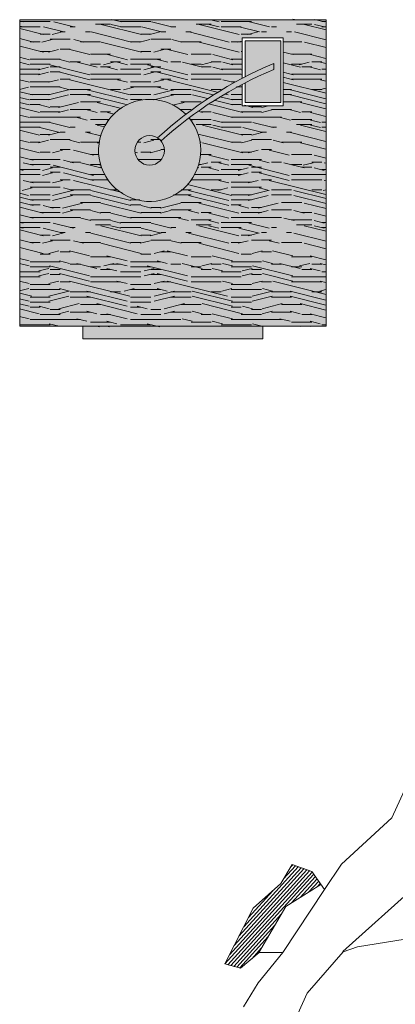
# Model space of a CAD drawing. Units: inches. Extents: x 1994 to 3075, y 3517 to 3950.
# Tile 34 of 58: x 1994.60824 to 1994.62882, y 3553.72103 to 3553.77497. Entities that reach past the tile are written whole.
import ezdxf

# ---------------------------------------------------------------- set-up
doc = ezdxf.new("R2010")
doc.units = ezdxf.units.IN
doc.layers.add('A-FURN-REFR', color=8, linetype='Continuous', lineweight=13)
doc.layers.add('A-FURN-REFR-PATT', color=8, linetype='Continuous', lineweight=13)

msp = doc.modelspace()

# ---------------------------------------------------------------- hatches: boundary and pattern name
at = {"layer": 'A-FURN-REFR-PATT'}
h = msp.add_hatch(color=256, dxfattribs=at)
h.paths.add_polyline_path([(1994.625025567844, 3553.774969762488), (1994.6082427092, 3553.774969762488), (1994.6082427092, 3553.758186903844), (1994.625025567844, 3553.758186903844)])
h.paths.add_polyline_path([(1994.617341065591, 3553.769785957469, -0.0420861834985648), (1994.620421545473, 3553.771753961409), (1994.620421545473, 3553.771757928811), (1994.620421545473, 3553.7739809259), (1994.622678150124, 3553.7739809259), (1994.622678150124, 3553.770259509415), (1994.620421545473, 3553.770259509415), (1994.620421545473, 3553.771423035513, 0.0395152736214861), (1994.617519187378, 3553.769589737948, -42.19598506456882)], flags=16)
h.paths.add_polyline_path([(1994.616171336827, 3553.767809896967, -1), (1994.614551403261, 3553.767809896967, -1)], flags=0)
h = msp.add_hatch(dxfattribs=at)
h.set_pattern_fill('LEGNO1', color=256, scale=0.005511811023622, style=0, pattern_type=2)
h.set_pattern_definition([(0, (2000.713136654079, 3549.954056641144), (0, 0.005511811023622), [0.0011023622047244, -0.0016535433070866, 0.0005511811023622, -0.0022047244094488]), (0, (2000.716994921796, 3549.95419443642), (0, 0.005511811023622), [0.0011023622047244, -0.0044094488188976]), (0, (2000.716443740693, 3549.954470026972), (0, 0.005511811023622), [0.0005511811023622, -0.0049606299212598]), (0, (2000.71341224463, 3549.954607822247), (0, 0.005511811023622), [0.0002755905511811, -0.0038582677165354, 0.0002755905511811, -0.0011023622047244]), (0, (2000.715341378489, 3549.954883412798), (0, 0.005511811023622), [0.0011023622047244, -0.0016535433070866, 0.0002755905511811, -0.0024803149606299]), (0, (2000.713963425733, 3549.955021208074), (0, 0.005511811023622), [0.0008267716535433, -0.0046850393700787]), (0, (2000.715341378489, 3549.955159003349), (0, 0.005511811023622), [0.0016535433070866, -0.0038582677165354]), (0, (2000.713687835181, 3549.955296798625), (0, 0.005511811023622), [0.0011023622047244, -0.0044094488188976]), (0, (2000.715892559591, 3549.955434593901), (0, 0.005511811023622), [0.002755905511811, -0.002755905511811]), (0, (2000.714239016284, 3549.955710184451), (0, 0.005511811023622), [0.0005511811023622, -0.0016535433070866, 0.0011023622047244, -0.0022047244094488]), (0, (2000.718097284, 3549.955847979727), (0, 0.005511811023622), [0.0011023622047244, -0.0044094488188976]), (0, (2000.716994921796, 3549.955985775002), (0, 0.005511811023622), [0.0005511811023622, -0.0049606299212598]), (0, (2000.715892559591, 3549.956123570279), (0, 0.005511811023622), [0.0005511811023622, -0.0049606299212598]), (0, (2000.713136654079, 3549.956261365553), (0, 0.005511811023622), [0.0011023622047244, -0.0044094488188976]), (0, (2000.715892559591, 3549.956399160829), (0, 0.005511811023622), [0.0011023622047244, -0.0044094488188976]), (0, (2000.715892559591, 3549.95667475138), (0, 0.005511811023622), [0.0011023622047244, -0.0011023622047244, 0.0011023622047244, -0.0022047244094488]), (0, (2000.714790197386, 3549.956950341932), (0, 0.005511811023622), [0.0005511811023622, -0.002755905511811, 0.0011023622047244, -0.0011023622047244]), (0, (2000.715892559591, 3549.957088137207), (0, 0.005511811023622), [0.0016535433070866, -0.0038582677165354]), (0, (2000.715892559591, 3549.957363727759), (0, 0.005511811023622), [0.0011023622047244, -0.0044094488188976]), (0, (2000.713687835181, 3549.957501523034), (0, 0.005511811023622), [0.0016535433070866, -0.0022047244094488, 0.0005511811023622, -0.0011023622047244]), (0, (2000.713687835181, 3549.957777113585), (0, 0.005511811023622), [0.002755905511811, -0.002755905511811]), (0, (2000.716994921796, 3549.957914908861), (0, 0.005511811023622), [0.0005511811023622, -0.0049606299212598]), (0, (2000.715341378489, 3549.958052704136), (0, 0.005511811023622), [0.0011023622047244, -0.0044094488188976]), (0, (2000.714239016284, 3549.958190499412), (0, 0.005511811023622), [0.0005511811023622, -0.0022047244094488, 0.0005511811023622, -0.0022047244094488]), (0, (2000.713687835181, 3549.958328294688), (0, 0.005511811023622), [0.0005511811023622, -0.0016535433070866, 0.0011023622047244, -0.0022047244094488]), (0, (2000.714790197386, 3549.958466089964), (0, 0.005511811023622), [0.0005511811023622, -0.002755905511811, 0.0005511811023622, -0.0016535433070866]), (0, (2000.715892559591, 3549.958603885239), (0, 0.005511811023622), [0.0016535433070866, -0.0038582677165354]), (0, (2000.713687835181, 3549.95887947579), (0, 0.005511811023622), [0.0011023622047244, -0.0044094488188976]), (0, (2000.716443740693, 3549.959017271066), (0, 0.005511811023622), [0.0005511811023622, -0.0049606299212598]), (0, (2000.717546102898, 3549.959155066341), (0, 0.005511811023622), [0.0005511811023622, -0.0049606299212598]), (14.03624347, (2000.716994921796, 3549.954470026972), (0.0055118110234648, -2.016e-13), [0.0005677165354331, -0.0221580619543307]), (14.03624347, (2000.717546102898, 3549.955710184451), (0.0055118110234648, -2.016e-13), [0.0005677165354331, -0.0221580619543307]), (14.03624347, (2000.716994921796, 3549.959017271066), (0.0055118110234648, -2.016e-13), [0.0005677165354331, -0.0221580619543307]), (14.03624347, (2000.715341378489, 3549.956950341932), (0.0055118110234648, -2.016e-13), [0.0005677165354331, -0.0221580619543307]), (14.03624347, (2000.716443740693, 3549.957777113585), (0.0055118110234648, -2.016e-13), [0.0005677165354331, -0.0221580619543307]), (14.03624347, (2000.716994921796, 3549.957363727759), (0.0055118110234648, -2.016e-13), [0.0005677165354331, -0.0221580619543307]), (14.03624347, (2000.714239016284, 3549.958328294688), (0.0055118110234648, -2.016e-13), [0.0005677165354331, -0.0221580619543307]), (14.03624347, (2000.716443740693, 3549.958052704136), (0.0055118110234648, -2.016e-13), [0.0005677165354331, -0.0221580619543307]), (14.03624347, (2000.717546102898, 3549.955985775002), (0.0055118110234648, -2.016e-13), [0.0011354330708661, -0.0215903454188977]), (14.03624347, (2000.716994921796, 3549.956399160829), (0.0055118110234648, -2.016e-13), [0.0011354330708661, -0.0215903454188977]), (14.03624347, (2000.716994921796, 3549.95667475138), (0.0055118110234648, -2.016e-13), [0.0011354330708661, -0.0215903454188977]), (165.96375653, (2000.715341378489, 3549.954883412798), (-0.0055118110234648, -2.016e-13), [0.0005677165354331, -0.0011354330708661, 0.0005677165354331, -0.0204549123480315]), (165.96375653, (2000.714239016284, 3549.955710184451), (-0.0055118110234648, -2.016e-13), [0.0005677165354331, -0.0221580619543307]), (165.96375653, (2000.714239016284, 3549.958190499412), (-0.0055118110234648, -2.016e-13), [0.0011354330708661, -0.0215903454188977]), (194.03624347, (2000.716994921796, 3549.95419443642), (-0.0055118110234648, 2.016e-13), [0.0005677165354331, -0.0221580619543307]), (345.96375653, (2000.718097284, 3549.95419443642), (0.0055118110234648, 2.016e-13), [0.0005677165354331, -0.0221580619543307]), (345.96375653, (2000.716443740693, 3549.956123570279), (0.0055118110234648, 2.016e-13), [0.0005677165354331, -0.0221580619543307]), (345.96375653, (2000.717546102898, 3549.957088137207), (0.0055118110234648, 2.016e-13), [0.0005677165354331, -0.0221580619543307]), (345.96375653, (2000.715341378489, 3549.957501523034), (0.0055118110234648, 2.016e-13), [0.0005677165354331, -0.0221580619543307]), (345.96375653, (2000.714790197386, 3549.958190499412), (0.0055118110234648, 2.016e-13), [0.0005677165354331, -0.0221580619543307]), (345.96375653, (2000.715341378489, 3549.958466089964), (0.0055118110234648, 2.016e-13), [0.0005677165354331, -0.0221580619543307]), (345.96375653, (2000.715341378489, 3549.957501523034), (0.0055118110234648, 2.016e-13), [0.0005677165354331, -0.0221580619543307]), (345.96375653, (2000.716994921796, 3549.958328294688), (0.0055118110234648, 2.016e-13), [0.0022708661417323, -0.0204549123480315]), (345.96375653, (2000.713687835181, 3549.954607822247), (0.0055118110234648, 2.016e-13), [0.0022708661417323, -0.0204549123480315]), (345.96375653, (2000.714239016284, 3549.955021208074), (0.0055118110234648, 2.016e-13), [0.0022708661417323, -0.0204549123480315]), (345.96375653, (2000.714790197386, 3549.955296798625), (0.0055118110234648, 2.016e-13), [0.0005677165354331, -0.0011354330708661, 0.0011354330708661, -0.0198871958125984]), (345.96375653, (2000.714790197386, 3549.955710184451), (0.0055118110234648, 2.016e-13), [0.0011354330708661, -0.0011354330708661, 0.0011354330708661, -0.0193194792771654]), (345.96375653, (2000.714239016284, 3549.956261365553), (0.0055118110234648, 2.016e-13), [0.0022708661417323, -0.0204549123480315]), (345.96375653, (2000.713687835181, 3549.95667475138), (0.0055118110234648, 2.016e-13), [0.0022708661417323, -0.0204549123480315]), (345.96375653, (2000.713687835181, 3549.956950341932), (0.0055118110234648, 2.016e-13), [0.0022708661417323, -0.0204549123480315]), (345.96375653, (2000.717546102898, 3549.958603885239), (0.0055118110234648, 2.016e-13), [0.0005677165354331, -0.0221580619543307]), (345.9637675300001, (2000.718097284, 3549.959155066341), (0.0055118110234647, 1.0583933e-09), [0.0011354330708661, -0.0215903454188977]), (345.9637675300001, (2000.714790197386, 3549.95887947579), (0.0055118110234647, 1.0583933e-09), [0.0011354330708661, -0.0215903454188977]), (345.96375753, (2000.714239016284, 3549.954056641144), (0.0055118110234648, 9.64008e-11), [0.0022708661417323, -0.0204549123480315]), (345.96375753, (2000.717546102898, 3549.957914908861), (0.0055118110234648, 9.64008e-11), [0.0017031496062992, -0.0210226288834646]), (345.96375753, (2000.718097284, 3549.957501523034), (0.0055118110234648, 9.64008e-11), [0.0034062992125984, -0.0193194792771654])])
h.paths.add_polyline_path([(1994.625025567844, 3553.774969762488), (1994.6082427092, 3553.774969762488), (1994.6082427092, 3553.758186903844), (1994.625025567844, 3553.758186903844)])
h.paths.add_polyline_path([(1994.617341065591, 3553.769785957469, -0.0420861834985648), (1994.620421545473, 3553.771753961409), (1994.620421545473, 3553.771757928811), (1994.620421545473, 3553.7739809259), (1994.622678150124, 3553.7739809259), (1994.622678150124, 3553.770259509415), (1994.620421545473, 3553.770259509415), (1994.620421545473, 3553.771423035513, 0.0395152736214861), (1994.617519187378, 3553.769589737948, -42.19598506456882)], flags=16)
h.paths.add_polyline_path([(1994.616171336827, 3553.767809896967, -1), (1994.614551403261, 3553.767809896967, -1)], flags=0)
msp.add_hatch(color=256, dxfattribs=at).paths.add_polyline_path([(1994.622545408993, 3553.773803717286), (1994.620598534099, 3553.773803717286), (1994.620598534099, 3553.771846057998, -0.0198106445216934), (1994.622160689546, 3553.772573101428), (1994.622160689546, 3553.772242175532, 0.0198106445217016), (1994.620598534099, 3553.771515132102), (1994.620598534099, 3553.770436718028), (1994.622545408993, 3553.770436718028)])
h = msp.add_hatch(color=256, dxfattribs=at)
h.dxf.hatch_style = 1
h.set_gradient(color1=(167, 169, 175), one_color=1, tint=1)
h.paths.add_polyline_path([(1994.622160689546, 3553.772242175532), (1994.622160689546, 3553.772573101428, 0.0875286051314429), (1994.61580001797, 3553.768490803852, -0.0763380806476787), (1994.615984121085, 3553.768327803648, -0.0846435149619904)])
h = msp.add_hatch(color=256, dxfattribs=at)
h.dxf.hatch_style = 1
h.set_gradient(color1=(37, 53, 157), color2=(142, 207, 230), tint=1, name='SPHERICAL')
h.paths.add_polyline_path([(1994.615361370044, 3553.76861986375, -0.1440580758931676), (1994.61580001797, 3553.768490803852, -0.0231477939795123), (1994.617341065591, 3553.769785957469, 42.19598506439846), (1994.617519187378, 3553.769589737948, 0.0228504078660832), (1994.615984121085, 3553.768327803648, -0.6355278128427492), (1994.615361370044, 3553.766999930184, -1)])
h = msp.add_hatch(color=256, dxfattribs=at)
h.dxf.hatch_style = 1
h.set_gradient(color1=(37, 40, 142), tint=1, name='INVSPHERICAL')
h.paths.add_polyline_path([(1994.615361370044, 3553.766999930184, 1), (1994.615361370044, 3553.76861986375, 1)])
h = msp.add_hatch(color=256, dxfattribs=at)
h.set_gradient(color1=(158, 155, 166), rotation=89.99999999999996, one_color=1, tint=1)
h.paths.add_polyline_path([(1994.621571871235, 3553.758186903844), (1994.611696405809, 3553.758186903844), (1994.611696405809, 3553.757480977518), (1994.621571871235, 3553.757480977518)])
h = msp.add_hatch(dxfattribs=at)
h.set_pattern_fill('ANSI31', color=256, scale=0.0011512997685247, angle=-0.070042260328277, style=0)
h.set_pattern_definition([(47.68516475108651, (1992.796339661784, 3550.732053809228), (0.0001019084019385, -0.0001119376326066), [])])
h.paths.add_polyline_path([(1994.622547310355, 3553.727648382726), (1994.623166281357, 3553.728690233518), (1994.624240091203, 3553.728300714385), (1994.624736786216, 3553.727596574512), (1994.622824334294, 3553.726401070794), (1994.621329302374, 3553.723835527964), (1994.62033175054, 3553.723016581393), (1994.619473848448, 3553.723244186343), (1994.621032750015, 3553.72629575506)])

# ---------------------------------------------------------------- linework, layer by layer
at = {"layer": 'A-FURN-REFR'}
for p, q in [((1994.6082427092, 3553.774969762488), (1994.625025567844, 3553.774969762488)), ((1994.6082427092, 3553.758186903844), (1994.6082427092, 3553.774969762488)), ((1994.625025567844, 3553.774969762488), (1994.625025567844, 3553.758186903844)), ((1994.622160689546, 3553.772573101428), (1994.622160689546, 3553.772242175532)), ((1994.625025567844, 3553.758186903844), (1994.6082427092, 3553.758186903844)), ((1994.628623063016, 3553.73124350498), (1994.629920631046, 3553.73408389857)), ((1994.625872840766, 3553.728712593434), (1994.628623063016, 3553.73124350498)), ((1994.622547310355, 3553.727648382726), (1994.623166281357, 3553.728690233518)), ((1994.623166281357, 3553.728690233518), (1994.624240091203, 3553.728300714385)), ((1994.624935463993, 3553.727314918886), (1994.625872840766, 3553.728712593434)), ((1994.624240091203, 3553.728300714385), (1994.624935463993, 3553.727314918886)), ((1994.630230800449, 3553.727784148941), (1994.625947466952, 3553.723933486272)), ((1994.621032750015, 3553.72629575506), (1994.622547310355, 3553.727648382726)), ((1994.624935463993, 3553.727314918886), (1994.622661748645, 3553.723864320283)), ((1994.624736786216, 3553.727596574512), (1994.622824334294, 3553.726401070794)), ((1994.619473848448, 3553.723244186343), (1994.621032750015, 3553.72629575506)), ((1994.622824334294, 3553.726401070794), (1994.621329302374, 3553.723835527964)), ((1994.629808700208, 3553.724679319563), (1994.626742683932, 3553.724183188604)), ((1994.626742683932, 3553.724183188604), (1994.625966017514, 3553.723900608345)), ((1994.621367929944, 3553.723867239515), (1994.62033175054, 3553.723016581393)), ((1994.621306022564, 3553.722205130184), (1994.622661748645, 3553.723864320283)), ((1994.622661748645, 3553.723864320283), (1994.621367929944, 3553.723867239515)), ((1994.625966017514, 3553.723900608345), (1994.623992462139, 3553.721652276177)), ((1994.62033175054, 3553.723016581393), (1994.619473848448, 3553.723244186343)), ((1994.620508096209, 3553.720894628283), (1994.621306022564, 3553.722205130184)), ((1994.623992462139, 3553.721652276177), (1994.623473435018, 3553.720516118564))]:
    msp.add_line(p, q, dxfattribs=at)
for points in [[(1994.620421545473, 3553.771753961409), (1994.620421545473, 3553.7739809259), (1994.622678150124, 3553.7739809259), (1994.622678150124, 3553.770259509415), (1994.620421545473, 3553.770259509415), (1994.620421545473, 3553.771423035513)], [(1994.620598534099, 3553.771846057998), (1994.620598534099, 3553.773803717286), (1994.622545408993, 3553.773803717286), (1994.622545408993, 3553.770436718028), (1994.620598534099, 3553.770436718028), (1994.620598534099, 3553.771515132102)], [(1994.620421545473, 3553.771753961409), (1994.620421545473, 3553.771757928811)], [(1994.620598534099, 3553.771846057998), (1994.620598534099, 3553.77185293988)]]:
    msp.add_lwpolyline(points, dxfattribs=at)
msp.add_lwpolyline([(1994.621571871235, 3553.757480977518), (1994.621571871235, 3553.758186903844), (1994.611696405809, 3553.758186903844), (1994.611696405809, 3553.757480977518)], close=True, dxfattribs=at)
msp.add_circle((1994.615361370044, 3553.767809896967), 0.0008099667829119, dxfattribs=at)
for centre, radius, start, end in [((1994.630550919859, 3553.752503729669), 0.0217526009365345, 112.6879237978252, 132.6970081735401), ((1994.630550919859, 3553.752172803773), 0.0217526009365345, 112.6879237978252, 132.0406587356917), ((1994.615361370044, 3553.767809896967), 0.002797143107239, 44.94734945639557, 39.51696962168485)]:
    msp.add_arc(centre, radius, start, end, dxfattribs=at)

doc.saveas('drawing.dxf')
